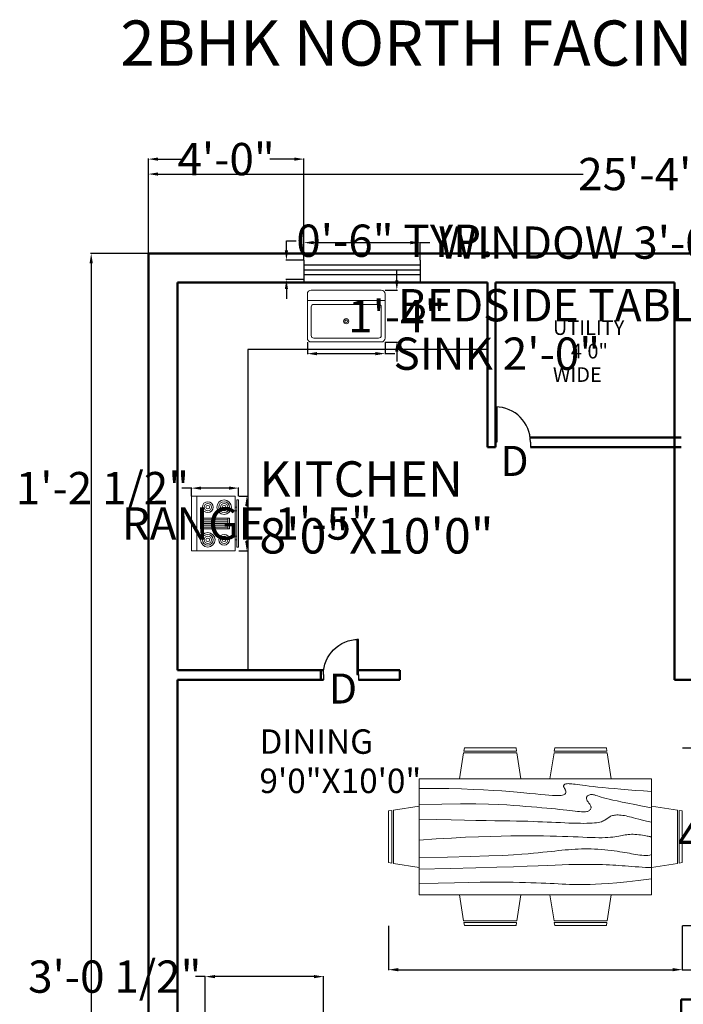
# Model space of a CAD drawing. Units: inches. Extents: x -35 to 382, y 867 to 1468.
# Tile 2 of 3: x -26 to 179, y 1163 to 1468. Entities that reach past the tile are written whole.
import ezdxf

# ---------------------------------------------------------------- set-up
doc = ezdxf.new("R2010")
doc.units = ezdxf.units.IN
doc.header["$MEASUREMENT"] = 0
for name, color, linetype, lineweight in [('A-ANNO-DIMS', 2, 'Continuous', 18), ('A-ANNO-TEXT', 7, 'Continuous', 25), ('A-AREA-IDEN', 7, 'Continuous', 25), ('A-DOOR', 3, 'Continuous', 25), ('A-EQPM', 8, 'Continuous', 18), ('A-FLOR-CASE', 32, 'Continuous', 25), ('A-FLOR-FIXT', 9, 'Continuous', 18), ('A-FURN', 9, 'Continuous', 18), ('A-GLAZ', 4, 'Continuous', 25), ('A-WALL', 7, 'Continuous', 50)]:
    doc.layers.add(name, color=color, linetype=linetype, lineweight=lineweight)
doc.styles.get("Standard").update_dxf_attribs({"font": 'arial.ttf'})
doc.dimstyles.get("Standard").update_dxf_attribs({"dimtxt": 10, "dimasz": 3, "dimexe": 0.18, "dimexo": 0.0625, "dimgap": 0.09, "dimtad": 0, "dimtih": 1, "dimtoh": 1, "dimdec": 0, "dimzin": 0, "dimdsep": 46, "dimlunit": 3, "dimtxsty": 'Standard', "dimcen": 0.09, "dimadec": 0, "dimazin": 0, "dimtfac": 1, "dimtdec": 0, "dimtofl": 0, "dimtmove": 0, "dimatfit": 3, "dimfxl": 1, "dimtolj": 1, "dimtzin": 0, "dimarcsym": 0})

# ---------------------------------------------------------------- blocks, each defined once
blk = doc.blocks.new('Sink-single - 30 in top')
blk.add_line((-15, -3.999996), (15, -3.999996))
for points in [[(-13.5, 0), (13.5, 0)], [(-15, -18.499996), (-15, -1.5)], [(15, -1.5), (15, -18.499996)], [(-13.5, -17.499996), (-13.5, -6.499996)], [(-12.5, -5.499996), (12.5, -5.499996)], [(13.5, -6.499996), (13.5, -17.499996)], [(12.5, -18.499996), (-12.5, -18.499996)], [(13.5, -19.999996), (-13.5, -19.999996)]]:
    blk.add_lwpolyline(points)
for radius in [1, 0.5]:
    blk.add_circle((0, -11.999996), radius)
for centre, radius, start, end in [((-13.5, -1.5), 1.5, 90, 180), ((13.5, -1.5), 1.5, 0, 90), ((-12.5, -6.499996), 1, 90, 180), ((12.5, -6.499996), 1, 0, 90), ((-13.5, -18.499996), 1.5, 180, 270), ((-12.5, -17.499996), 1, 180, 270), ((12.5, -17.499996), 1, 270, 0), ((13.5, -18.499996), 1.5, 270, 0)]:
    blk.add_arc(centre, radius, start, end)
blk = doc.blocks.new('Range-Oven - 30 in top')
for p, q in [((0, -3), (30, -3)), ((12, -6), (18, -6)), ((13, -20), (13, -6)), ((14, -6), (14, -20)), ((15, -20), (15, -6)), ((16, -6), (16, -20)), ((17, -20), (17, -6)), ((18, -20), (12, -20)), ((6, -24), (6, -25)), ((8, -25), (8, -24)), ((22, -25), (22, -24)), ((24, -24), (24, -25))]:
    blk.add_line(p, q)
for points in [[(0, -24), (0, 0), (30, 0), (30, -24)], [(12, -21), (12, -5), (18, -5), (18, -21)], [(2, -26), (2, -25), (28, -25), (28, -26)]]:
    blk.add_lwpolyline(points, close=True)
for centre, radius in [((6, -9), 4), ((6, -9), 3), ((6, -9), 2), ((6, -9), 1), ((24, -9), 3), ((24, -9), 2), ((24, -9), 1), ((6, -18), 3), ((6, -18), 2), ((24, -18), 4), ((24, -18), 3), ((24, -18), 2), ((6, -18), 1), ((24, -18), 1)]:
    blk.add_circle(centre, radius)
blk = doc.blocks.new('*U9')
for p, q in [((0, 0), (0, -6)), ((40, 0), (40, -6))]:
    blk.add_line(p, q)
blk.add_lwpolyline([(0, 0), (0, 40), (1.75, 40), (1.75, 0)], close=True)
blk.add_arc((0, 0), 40, 0, 90)
blk = doc.blocks.new('Dining Set - 36 x 72 in.')
for p, q in [((-22, 27.5), (-22.1562, 26.50042)), ((-22, 27.5), (-6, 27.5)), ((-5.8437, 26.49966), (-6, 27.5)), ((6, 27.5), (5.8438, 26.50042)), ((6, 27.5), (22, 27.5)), ((22.1563, 26.49966), (22, 27.5)), ((-22.2343, 26.00059), (-23.4847, 17.99762)), ((-22.2304, 26), (-5.7608, 26)), ((-5.8416, 26.5), (-22.1534, 26.5)), ((-4.5152, 17.99762), (-5.7655, 25.99926)), ((5.7657, 26.00059), (4.5153, 17.99762)), ((5.7696, 26), (22.2392, 26)), ((22.1584, 26.5), (5.8466, 26.5)), ((23.4848, 17.99762), (22.2345, 25.99926)), ((36, 18), (-36, 18)), ((-36, 18), (-36, -18)), ((36, -18), (36, 18)), ((-44.0006, 8.23428), (-35.9976, 9.48474)), ((44.0006, 8.23428), (35.9976, 9.48474)), ((-45.5, 8), (-44.5004, 8.15617)), ((-45.5, 8), (-45.5, -8)), ((-44.5, -8.15843), (-44.5, 8.15338)), ((-44, 8.23041), (-44, -8.23915)), ((44, 8.23041), (44, -8.23915)), ((44.5, -8.15843), (44.5, 8.15338)), ((45.5, 8), (44.5005, 8.15617)), ((45.5, 8), (45.5, -8)), ((-44.4997, -8.15631), (-45.5, -8)), ((-35.9976, -9.48476), (-43.9993, -8.2345)), ((35.9976, -9.48476), (43.9993, -8.2345)), ((44.4997, -8.15631), (45.5, -8)), ((-36, -18), (36, -18)), ((-22.2343, -26.0006), (-23.4847, -17.99762)), ((-4.5152, -17.99762), (-5.7655, -25.99928)), ((5.7657, -26.0006), (4.5153, -17.99762)), ((23.4848, -17.99762), (22.2345, -25.99928)), ((-22.2304, -26), (-5.7608, -26)), ((-22, -27.5), (-22.1562, -26.50044)), ((-5.8416, -26.5), (-22.1534, -26.5)), ((-5.8437, -26.49967), (-6, -27.5)), ((5.7696, -26), (22.2392, -26)), ((6, -27.5), (5.8438, -26.50044)), ((22.1584, -26.5), (5.8466, -26.5)), ((22.1563, -26.49967), (22, -27.5)), ((-22, -27.5), (-6, -27.5)), ((6, -27.5), (22, -27.5))]:
    blk.add_line(p, q)
for points in [[(-36, 15), (-31.1772, 14.97754), (-26.8079, 14.91406), (-22.8538, 14.81543), (-19.276, 14.6875), (-16.0362, 14.53613), (-13.0957, 14.36718), (-10.4159, 14.18652), (-7.9583, 14), (-5.6904, 13.81315), (-3.6035, 13.63021), (-1.6954, 13.45508), (0.0365, 13.29166), (1.5945, 13.14388), (2.9811, 13.01562), (4.1988, 12.9108), (5.25, 12.83333), (6.1393, 12.78613), (6.8802, 12.76823), (7.4883, 12.77767), (7.9792, 12.8125), (8.3685, 12.87077), (8.6719, 12.95052), (8.9049, 13.0498), (9.0833, 13.16666), (9.2205, 13.29899), (9.3216, 13.44401), (9.3895, 13.59879), (9.4271, 13.76041), (9.4373, 13.92594), (9.4232, 14.09245), (9.3875, 14.257), (9.3333, 14.41666), (9.2638, 14.56917), (9.1836, 14.71484), (9.0975, 14.85465), (9.0104, 14.98958), (8.9272, 15.1206), (8.8529, 15.2487), (8.7922, 15.37483), (8.75, 15.5), (8.7305, 15.62467), (8.7344, 15.74739), (8.7617, 15.86621), (8.8125, 15.97916), (8.8867, 16.08431), (8.9844, 16.17968), (9.1055, 16.26334), (9.25, 16.33333), (9.4189, 16.38802), (9.6172, 16.42708), (9.8506, 16.45052), (10.125, 16.45833), (10.4463, 16.45052), (10.8203, 16.42708), (11.2529, 16.38802), (11.75, 16.33333), (12.3184, 16.26318), (12.9694, 16.17838), (13.7151, 16.07991), (14.5677, 15.96875), (15.5395, 15.84586), (16.6426, 15.71224), (17.8893, 15.56884), (19.2917, 15.41666), (20.859, 15.25667), (22.5879, 15.08984), (24.4721, 14.91715), (26.5052, 14.73958), (28.6809, 14.5581), (30.9929, 14.3737), (33.4347, 14.18733), (36, 14)], [(-36, 10), (-28.9766, 10.14274), (-23.1725, 10.20442), (-18.4241, 10.19775), (-14.5677, 10.13541), (-11.4399, 10.03011), (-8.877, 9.89453), (-6.7154, 9.74137), (-4.7917, 9.58333), (-2.9698, 9.43082), (-1.2246, 9.28515), (0.4415, 9.14534), (2.026, 9.01041), (3.5266, 8.87939), (4.9408, 8.7513), (6.266, 8.62516), (7.5, 8.5), (8.6411, 8.37549), (9.6914, 8.2539), (10.6538, 8.13818), (11.5312, 8.03125), (12.3267, 7.93603), (13.043, 7.85547), (13.6831, 7.79248), (14.25, 7.75), (14.7471, 7.7303), (15.1797, 7.73307), (15.5537, 7.75732), (15.875, 7.80208), (16.1494, 7.86637), (16.3828, 7.94922), (16.5811, 8.04964), (16.75, 8.16666), (16.8944, 8.29915), (17.0143, 8.44531), (17.1089, 8.60319), (17.1771, 8.77083), (17.218, 8.94629), (17.2305, 9.1276), (17.2137, 9.31282), (17.1667, 9.5), (17.0895, 9.6875), (16.987, 9.875), (16.8649, 10.0625), (16.7292, 10.25), (16.5856, 10.4375), (16.4401, 10.625), (16.2985, 10.8125), (16.1667, 11), (16.05, 11.18733), (15.9518, 11.3737), (15.8752, 11.5581), (15.8229, 11.73958), (15.798, 11.91715), (15.8034, 12.08984), (15.842, 12.25667), (15.9167, 12.41666), (16.0295, 12.56836), (16.1784, 12.70833), (16.3605, 12.83268), (16.5729, 12.9375), (16.8127, 13.01888), (17.0768, 13.07291), (17.3625, 13.0957), (17.6667, 13.08333), (17.9894, 13.03312), (18.3418, 12.94726), (18.7382, 12.82918), (19.1927, 12.68229), (19.7195, 12.51001), (20.3327, 12.31575), (21.0465, 12.10294), (21.875, 11.875), (22.8357, 11.63354), (23.959, 11.37304), (25.2786, 11.08618), (26.8282, 10.76562), (28.6414, 10.40405), (30.752, 9.99414), (33.1936, 9.52856), (36, 9)], [(-36, 5.5), (-30.7157, 5.3348), (-26.069, 5.20963), (-21.9946, 5.11767), (-18.4271, 5.05208), (-15.3009, 5.00602), (-12.5508, 4.97265), (-10.1112, 4.94515), (-7.9167, 4.91666), (-5.909, 4.88167), (-4.0586, 4.83984), (-2.3429, 4.79215), (-0.7396, 4.73958), (0.7739, 4.6831), (2.22, 4.6237), (3.6213, 4.56233), (5, 4.5), (6.373, 4.43782), (7.7344, 4.3776), (9.0723, 4.32129), (10.375, 4.27083), (11.6309, 4.22819), (12.8281, 4.19531), (13.9551, 4.17415), (15, 4.16666), (15.954, 4.17448), (16.819, 4.19791), (17.6001, 4.23698), (18.3021, 4.29166), (18.9299, 4.36198), (19.4883, 4.44791), (19.9823, 4.54948), (20.4167, 4.66666), (20.7969, 4.79899), (21.1302, 4.94401), (21.4245, 5.09879), (21.6875, 5.26041), (21.9271, 5.42594), (22.1511, 5.59245), (22.3672, 5.757), (22.5834, 5.91666), (22.8065, 6.06868), (23.0404, 6.21093), (23.2879, 6.34147), (23.5521, 6.45833), (23.8358, 6.55957), (24.142, 6.64323), (24.4735, 6.70735), (24.8334, 6.75), (25.2235, 6.76969), (25.642, 6.76692), (26.0858, 6.74267), (26.5521, 6.69791), (27.0379, 6.63362), (27.5404, 6.55078), (28.0565, 6.45036), (28.5834, 6.33333), (29.1242, 6.19987), (29.7071, 6.04687), (30.3661, 5.87044), (31.1354, 5.66666), (32.0493, 5.43164), (33.142, 5.16146), (34.4475, 4.85221), (36, 4.5)], [(-36, -1), (-30.7915, -0.6591), (-26.0195, -0.38216), (-21.6519, -0.16284), (-17.6563, 0.00521), (-14.0005, 0.12833), (-10.6523, 0.21289), (-7.5796, 0.26522), (-4.75, 0.29166), (-2.134, 0.29793), (0.2878, 0.28711), (2.5317, 0.26163), (4.6146, 0.22396), (6.5529, 0.17651), (8.3633, 0.12174), (10.0623, 0.06209), (11.6667, 0), (13.1899, -0.06201), (14.6341, -0.1211), (15.9982, -0.17432), (17.2813, -0.21875), (18.4823, -0.25147), (19.6003, -0.26953), (20.6343, -0.27002), (21.5834, -0.25), (22.4481, -0.20768), (23.2357, -0.14584), (23.9549, -0.06836), (24.6146, 0.02083), (25.2235, 0.11784), (25.7904, 0.21875), (26.3241, 0.31966), (26.8334, 0.41666), (27.3265, 0.50618), (27.8099, 0.58593), (28.2894, 0.65397), (28.7709, 0.70833), (29.2601, 0.74707), (29.763, 0.76823), (30.2855, 0.76985), (30.8334, 0.75), (31.4088, 0.70784), (31.9994, 0.64713), (32.589, 0.57275), (33.1615, 0.48958), (33.7008, 0.4025), (34.1908, 0.3164), (34.6153, 0.23616), (34.9584, 0.16666), (35.2099, 0.11165), (35.3848, 0.07031), (35.504, 0.04069), (35.5886, 0.02083), (35.6594, 0.00879), (35.7377, 0.0026), (35.8442, 0.00032), (36, 0)], [(-36, -6.5), (-27.1843, -6.31267), (-20.084, -6.1263), (-14.469, -5.9419), (-10.1094, -5.76042), (-6.7752, -5.58285), (-4.2363, -5.41016), (-2.2629, -5.24333), (-0.625, -5.08334), (0.8708, -4.93099), (2.2715, -4.78646), (3.5872, -4.64974), (4.8281, -4.52084), (6.0046, -4.39974), (7.127, -4.28646), (8.2053, -4.18099), (9.25, -4.08334), (10.2705, -3.99382), (11.2734, -3.91407), (12.2647, -3.84603), (13.25, -3.79167), (14.2354, -3.75293), (15.2266, -3.73177), (16.2295, -3.73015), (17.25, -3.75), (18.2912, -3.79248), (19.3451, -3.85547), (20.4009, -3.93604), (21.4479, -4.03125), (22.4754, -4.13819), (23.4727, -4.25391), (24.4289, -4.37549), (25.3334, -4.5), (26.1785, -4.62492), (26.9694, -4.74935), (27.7145, -4.87281), (28.4219, -4.99479), (29.1, -5.11483), (29.7572, -5.23242), (30.4016, -5.34709), (31.0417, -5.45834), (31.6837, -5.56437), (32.3262, -5.65821), (32.9658, -5.73153), (33.599, -5.77604), (34.2224, -5.78345), (34.8327, -5.74545), (35.4264, -5.65373), (36, -5.5)], [(-36, -10), (-26.4022, -9.81299), (-18.4675, -9.62891), (-11.9839, -9.45069), (-6.7396, -9.28125), (-2.5226, -9.12354), (0.8789, -8.98047), (3.6769, -8.85498), (6.0833, -8.75), (8.2767, -8.66765), (10.3021, -8.60677), (12.1712, -8.56543), (13.8958, -8.54167), (15.4876, -8.53353), (16.9583, -8.53907), (18.3197, -8.55632), (19.5834, -8.58334), (20.7616, -8.61841), (21.8685, -8.66081), (22.9188, -8.71004), (23.9271, -8.76563), (24.9081, -8.82707), (25.8763, -8.89388), (26.8465, -8.96558), (27.8334, -9.04167), (28.8474, -9.12118), (29.8828, -9.20117), (30.93, -9.27824), (31.9792, -9.34896), (33.0205, -9.40991), (34.0443, -9.45768), (35.0407, -9.48885), (36, -9.5)], [(-36, -14.5), (-30.0881, -14.33513), (-25.0332, -14.21224), (-20.7312, -14.12647), (-17.0781, -14.07292), (-13.97, -14.04671), (-11.3027, -14.04297), (-8.9724, -14.05681), (-6.875, -14.08334), (-4.9224, -14.11833), (-3.0905, -14.16016), (-1.3709, -14.20785), (0.2448, -14.26042), (1.7647, -14.3169), (3.1973, -14.3763), (4.5507, -14.43767), (5.8333, -14.5), (7.0554, -14.5621), (8.235, -14.62175), (9.3922, -14.67652), (10.5469, -14.72396), (11.7192, -14.76164), (12.929, -14.78711), (14.1965, -14.79794), (15.5417, -14.79167), (16.9933, -14.76424), (18.6152, -14.70508), (20.4804, -14.60197), (22.6615, -14.44271), (25.2312, -14.21509), (28.2624, -13.9069), (31.8277, -13.50594), (36, -13)]]:
    blk.add_lwpolyline(points)
blk = doc.blocks.new('Window - Wood Frame 36 in. Wide plan')
for p, q in [((0, 6), (0, 0)), ((0, 4.5), (36, 4.5)), ((36, 6), (36, 0)), ((0, 3), (36, 3)), ((0, 1.5), (36, 1.5))]:
    blk.add_line(p, q)
blk = doc.blocks.new('*D15')
at = {"layer": 'A-ANNO-DIMS', "color": 0, "lineweight": -2, "transparency": 16777216}
for p, q in [((13.52, 1395.38), (13.52, 1420.11)), ((16.52, 1419.93), (148.17, 1419.93)), ((314.52, 1419.93), (182.87, 1419.93)), ((317.52, 1395.38), (317.52, 1420.11))]:
    blk.add_line(p, q, dxfattribs=at)
at = {"layer": 'A-ANNO-DIMS', "color": 0, "transparency": 16777216}
for points in [[(16.52, 1420.43), (16.52, 1419.43), (13.52, 1419.93)], [(314.52, 1420.43), (314.52, 1419.43), (317.52, 1419.93)]]:
    blk.add_solid(points, dxfattribs=at)
at = {"layer": 'Defpoints', "color": 0, "transparency": 16777216}
for p in [(317.52, 1419.93), (13.52, 1395.31), (317.52, 1395.31)]:
    blk.add_point(p, dxfattribs=at)
at = {"layer": 'A-ANNO-DIMS', "color": 0, "transparency": 16777216, "insert": (165.52, 1419.93), "char_height": 10, "attachment_point": 5}
blk.add_mtext('\\A1;25\'-4"', dxfattribs=at)
blk = doc.blocks.new('*D16')
at = {"layer": 'A-ANNO-DIMS', "color": 0, "lineweight": -2, "transparency": 16777216}
for p, q in [((13.46, 1395.31), (-4.36, 1395.31)), ((-4.18, 1392.31), (-4.18, 1158.51)), ((-4.18, 914.31), (-4.18, 1148.12)), ((13.46, 911.31), (-4.36, 911.31))]:
    blk.add_line(p, q, dxfattribs=at)
at = {"layer": 'A-ANNO-DIMS', "color": 0, "transparency": 16777216}
for points in [[(-4.68, 1392.31), (-3.68, 1392.31), (-4.18, 1395.31)], [(-4.68, 914.31), (-3.68, 914.31), (-4.18, 911.31)]]:
    blk.add_solid(points, dxfattribs=at)
at = {"layer": 'Defpoints', "color": 0, "transparency": 16777216}
for p in [(13.52, 1395.31), (-4.18, 911.31), (13.52, 911.31)]:
    blk.add_point(p, dxfattribs=at)
at = {"layer": 'A-ANNO-DIMS', "color": 0, "transparency": 16777216, "insert": (-4.18, 1153.31), "char_height": 10, "attachment_point": 5}
blk.add_mtext('\\A1;40\'-4"', dxfattribs=at)
blk = doc.blocks.new('*D18')
at = {"layer": 'A-ANNO-DIMS', "color": 0, "lineweight": -2, "transparency": 16777216}
for p, q in [((61.69, 1393.35), (61.69, 1398.87)), ((64.69, 1398.69), (94.69, 1398.69)), ((97.69, 1393.35), (97.69, 1398.87)), ((97.69, 1398.69), (100.69, 1398.69))]:
    blk.add_line(p, q, dxfattribs=at)
at = {"layer": 'A-ANNO-DIMS', "color": 0, "transparency": 16777216}
for points in [[(64.69, 1399.19), (64.69, 1398.19), (61.69, 1398.69)], [(94.69, 1399.19), (94.69, 1398.19), (97.69, 1398.69)]]:
    blk.add_solid(points, dxfattribs=at)
at = {"layer": 'Defpoints', "color": 0, "transparency": 16777216}
for p in [(97.69, 1398.69), (61.69, 1393.29), (97.69, 1393.29)]:
    blk.add_point(p, dxfattribs=at)
at = {"layer": 'A-ANNO-DIMS', "color": 0, "transparency": 16777216, "insert": (164.05, 1398.69), "char_height": 10, "attachment_point": 5}
blk.add_mtext('\\A1;WINDOW 3\'-0" TYP.', dxfattribs=at)
blk = doc.blocks.new('*D19')
at = {"layer": 'A-ANNO-DIMS', "color": 0, "lineweight": -2, "transparency": 16777216}
for p, q in [((56.29, 1396.29), (56.29, 1399.29)), ((56.29, 1399.29), (59.29, 1399.29)), ((61.63, 1393.29), (56.11, 1393.29)), ((61.63, 1387.29), (56.11, 1387.29)), ((56.29, 1384.29), (56.29, 1381.29))]:
    blk.add_line(p, q, dxfattribs=at)
at = {"layer": 'A-ANNO-DIMS', "color": 0, "transparency": 16777216}
for points in [[(55.79, 1396.29), (56.79, 1396.29), (56.29, 1393.29)], [(55.79, 1384.29), (56.79, 1384.29), (56.29, 1387.29)]]:
    blk.add_solid(points, dxfattribs=at)
at = {"layer": 'Defpoints', "color": 0, "transparency": 16777216}
for p in [(56.29, 1393.29), (61.69, 1393.29), (61.69, 1387.29)]:
    blk.add_point(p, dxfattribs=at)
at = {"layer": 'A-ANNO-DIMS', "color": 0, "transparency": 16777216, "insert": (89.86, 1399.29), "char_height": 10, "attachment_point": 5}
blk.add_mtext('\\A1;0\'-6" TYP.', dxfattribs=at)
blk = doc.blocks.new('*D22')
at = {"layer": 'A-ANNO-DIMS', "color": 0, "lineweight": -2, "transparency": 16777216}
for p, q in [((286.27, 1379.31), (283.27, 1379.31)), ((286.27, 1377.52), (286.27, 1379.49)), ((295.61, 1379.31), (289.27, 1379.31)), ((298.61, 1377.52), (298.61, 1379.49))]:
    blk.add_line(p, q, dxfattribs=at)
at = {"layer": 'A-ANNO-DIMS', "color": 0, "transparency": 16777216}
for points in [[(289.27, 1379.81), (289.27, 1378.81), (286.27, 1379.31)], [(295.61, 1379.81), (295.61, 1378.81), (298.61, 1379.31)]]:
    blk.add_solid(points, dxfattribs=at)
at = {"layer": 'Defpoints', "color": 0, "transparency": 16777216}
for p in [(286.27, 1379.31), (286.27, 1377.46), (298.61, 1377.46)]:
    blk.add_point(p, dxfattribs=at)
at = {"layer": 'A-ANNO-DIMS', "color": 0, "transparency": 16777216, "insert": (184.6, 1379.31), "char_height": 10, "attachment_point": 5}
blk.add_mtext('\\A1;BEDSIDE TABLE 1\'-0 1/2" TYP.', dxfattribs=at)
blk = doc.blocks.new('*D31')
at = {"layer": 'A-ANNO-DIMS', "color": 0, "lineweight": -2, "transparency": 16777216}
for p, q in [((31.15, 1171.39), (28.15, 1171.39)), ((31.15, 1158.85), (31.15, 1171.57)), ((64.82, 1171.39), (34.15, 1171.39)), ((67.82, 1158.85), (67.82, 1171.57))]:
    blk.add_line(p, q, dxfattribs=at)
at = {"layer": 'A-ANNO-DIMS', "color": 0, "transparency": 16777216}
for points in [[(34.15, 1171.89), (34.15, 1170.89), (31.15, 1171.39)], [(64.82, 1171.89), (64.82, 1170.89), (67.82, 1171.39)]]:
    blk.add_solid(points, dxfattribs=at)
at = {"layer": 'Defpoints', "color": 0, "transparency": 16777216}
for p in [(31.15, 1171.39), (31.15, 1158.79), (67.82, 1158.79)]:
    blk.add_point(p, dxfattribs=at)
at = {"layer": 'A-ANNO-DIMS', "color": 0, "transparency": 16777216, "insert": (3.12, 1171.39), "char_height": 10, "attachment_point": 5}
blk.add_mtext('\\A1;3\'-0 1/2"', dxfattribs=at)
blk = doc.blocks.new('*D32')
at = {"layer": 'A-ANNO-DIMS', "color": 0, "lineweight": -2, "transparency": 16777216}
for p, q in [((62.77, 1367.86), (62.77, 1364.13)), ((86.86, 1367.86), (86.86, 1364.13)), ((65.77, 1364.31), (83.86, 1364.31)), ((86.86, 1364.31), (89.86, 1364.31))]:
    blk.add_line(p, q, dxfattribs=at)
at = {"layer": 'A-ANNO-DIMS', "color": 0, "transparency": 16777216}
for points in [[(65.77, 1364.81), (65.77, 1363.81), (62.77, 1364.31)], [(83.86, 1364.81), (83.86, 1363.81), (86.86, 1364.31)]]:
    blk.add_solid(points, dxfattribs=at)
at = {"layer": 'Defpoints', "color": 0, "transparency": 16777216}
for p in [(62.77, 1367.92), (86.86, 1367.92), (86.86, 1364.31)]:
    blk.add_point(p, dxfattribs=at)
at = {"layer": 'A-ANNO-DIMS', "color": 0, "transparency": 16777216, "insert": (121.46, 1364.31), "char_height": 10, "attachment_point": 5}
blk.add_mtext('\\A1;SINK 2\'-0"', dxfattribs=at)
blk = doc.blocks.new('*D33')
at = {"layer": 'A-ANNO-DIMS', "color": 0, "lineweight": -2, "transparency": 16777216}
for p, q in [((90.47, 1386.98), (90.47, 1389.98)), ((86.92, 1383.98), (90.65, 1383.98)), ((86.92, 1367.92), (90.65, 1367.92)), ((90.47, 1364.92), (90.47, 1361.92))]:
    blk.add_line(p, q, dxfattribs=at)
at = {"layer": 'A-ANNO-DIMS', "color": 0, "transparency": 16777216}
for points in [[(89.97, 1386.98), (90.97, 1386.98), (90.47, 1383.98)], [(89.97, 1364.92), (90.97, 1364.92), (90.47, 1367.92)]]:
    blk.add_solid(points, dxfattribs=at)
at = {"layer": 'Defpoints', "color": 0, "transparency": 16777216}
for p in [(86.86, 1383.98), (90.47, 1383.98), (86.86, 1367.92)]:
    blk.add_point(p, dxfattribs=at)
at = {"layer": 'A-ANNO-DIMS', "color": 0, "transparency": 16777216, "insert": (90.47, 1375.95), "char_height": 10, "attachment_point": 5}
blk.add_mtext('\\A1;1\'-4"', dxfattribs=at)
blk = doc.blocks.new('*D34')
at = {"layer": 'A-ANNO-DIMS', "color": 0, "lineweight": -2, "transparency": 16777216}
for p, q in [((41.54, 1320.14), (44.19, 1320.14)), ((44.01, 1317.14), (44.01, 1316.98)), ((44.01, 1306.29), (44.01, 1306.45)), ((41.54, 1303.29), (44.19, 1303.29))]:
    blk.add_line(p, q, dxfattribs=at)
at = {"layer": 'A-ANNO-DIMS', "color": 0, "transparency": 16777216}
for points in [[(43.51, 1317.14), (44.51, 1317.14), (44.01, 1320.14)], [(43.51, 1306.29), (44.51, 1306.29), (44.01, 1303.29)]]:
    blk.add_solid(points, dxfattribs=at)
at = {"layer": 'Defpoints', "color": 0, "transparency": 16777216}
for p in [(41.48, 1320.14), (44.01, 1320.14), (41.48, 1303.29)]:
    blk.add_point(p, dxfattribs=at)
at = {"layer": 'A-ANNO-DIMS', "color": 0, "transparency": 16777216, "insert": (44.01, 1311.71), "char_height": 10, "attachment_point": 5}
blk.add_mtext('\\A1;RANGE 1\'-5"', dxfattribs=at)
blk = doc.blocks.new('*D35')
at = {"layer": 'A-ANNO-DIMS', "color": 0, "lineweight": -2, "transparency": 16777216}
for p, q in [((26.88, 1322.67), (23.88, 1322.67)), ((26.88, 1320.2), (26.88, 1322.85)), ((38.48, 1322.67), (29.88, 1322.67)), ((41.48, 1320.2), (41.48, 1322.85))]:
    blk.add_line(p, q, dxfattribs=at)
at = {"layer": 'A-ANNO-DIMS', "color": 0, "transparency": 16777216}
for points in [[(29.88, 1323.17), (29.88, 1322.17), (26.88, 1322.67)], [(38.48, 1323.17), (38.48, 1322.17), (41.48, 1322.67)]]:
    blk.add_solid(points, dxfattribs=at)
at = {"layer": 'Defpoints', "color": 0, "transparency": 16777216}
for p in [(26.88, 1322.67), (26.88, 1320.14), (41.48, 1320.14)]:
    blk.add_point(p, dxfattribs=at)
at = {"layer": 'A-ANNO-DIMS', "color": 0, "transparency": 16777216, "insert": (-0.69, 1322.67), "char_height": 10, "attachment_point": 5}
blk.add_mtext('\\A1;1\'-2 1/2"', dxfattribs=at)
blk = doc.blocks.new('*D36')
at = {"layer": 'A-ANNO-DIMS', "color": 0, "lineweight": -2, "transparency": 16777216}
for p, q in [((87.91, 1187.13), (87.91, 1173.36)), ((178.91, 1187.13), (178.91, 1173.36)), ((90.91, 1173.54), (175.91, 1173.54)), ((178.91, 1173.54), (181.91, 1173.54))]:
    blk.add_line(p, q, dxfattribs=at)
at = {"layer": 'A-ANNO-DIMS', "color": 0, "transparency": 16777216}
for points in [[(90.91, 1174.04), (90.91, 1173.04), (87.91, 1173.54)], [(175.91, 1174.04), (175.91, 1173.04), (178.91, 1173.54)]]:
    blk.add_solid(points, dxfattribs=at)
at = {"layer": 'Defpoints', "color": 0, "transparency": 16777216}
for p in [(87.91, 1187.19), (178.91, 1187.19), (178.91, 1173.54)]:
    blk.add_point(p, dxfattribs=at)
at = {"layer": 'A-ANNO-DIMS', "color": 0, "transparency": 16777216, "insert": (236.96, 1173.54), "char_height": 10, "attachment_point": 5}
blk.add_mtext('\\A1;DINING SET 7\'-7"', dxfattribs=at)
blk = doc.blocks.new('*D37')
at = {"layer": 'A-ANNO-DIMS', "color": 0, "lineweight": -2, "transparency": 16777216}
for p, q in [((178.97, 1242.19), (192.74, 1242.19)), ((192.56, 1239.19), (192.56, 1219.78)), ((192.56, 1190.19), (192.56, 1209.6)), ((178.97, 1187.19), (192.74, 1187.19))]:
    blk.add_line(p, q, dxfattribs=at)
at = {"layer": 'A-ANNO-DIMS', "color": 0, "transparency": 16777216}
for points in [[(192.06, 1239.19), (193.06, 1239.19), (192.56, 1242.19)], [(192.06, 1190.19), (193.06, 1190.19), (192.56, 1187.19)]]:
    blk.add_solid(points, dxfattribs=at)
at = {"layer": 'Defpoints', "color": 0, "transparency": 16777216}
for p in [(178.91, 1242.19), (192.56, 1242.19), (178.91, 1187.19)]:
    blk.add_point(p, dxfattribs=at)
at = {"layer": 'A-ANNO-DIMS', "color": 0, "transparency": 16777216, "insert": (192.56, 1214.69), "char_height": 10, "attachment_point": 5}
blk.add_mtext('\\A1;4\'-7"', dxfattribs=at)
blk = doc.blocks.new('*D47')
at = {"layer": 'A-ANNO-DIMS', "color": 0, "lineweight": -2, "transparency": 16777216}
for p, q in [((13.52, 1395.38), (13.52, 1424.74)), ((16.52, 1424.56), (24.02, 1424.56)), ((58.69, 1424.56), (51.19, 1424.56)), ((61.69, 1395.38), (61.69, 1424.74))]:
    blk.add_line(p, q, dxfattribs=at)
at = {"layer": 'A-ANNO-DIMS', "color": 0, "transparency": 16777216}
for points in [[(16.52, 1425.06), (16.52, 1424.06), (13.52, 1424.56)], [(58.69, 1425.06), (58.69, 1424.06), (61.69, 1424.56)]]:
    blk.add_solid(points, dxfattribs=at)
at = {"layer": 'Defpoints', "color": 0, "transparency": 16777216}
for p in [(61.69, 1424.56), (13.52, 1395.31), (61.69, 1395.31)]:
    blk.add_point(p, dxfattribs=at)
at = {"layer": 'A-ANNO-DIMS', "color": 0, "transparency": 16777216, "insert": (37.61, 1424.56), "char_height": 10, "attachment_point": 5}
blk.add_mtext('\\A1;4\'-0"', dxfattribs=at)

msp = doc.modelspace()

# ---------------------------------------------------------------- linework, layer by layer
at = {"layer": 'A-FLOR-CASE'}
for p, q in [((118.52, 1365.57), (44.34, 1365.57)), ((44.34, 1365.57), (44.34, 1266.31))]:
    msp.add_line(p, q, dxfattribs=at)
at = {"layer": 'A-GLAZ'}
for p, q in [((61.69, 1393.29), (61.69, 1395.31)), ((97.69, 1393.29), (97.69, 1395.31)), ((61.69, 1387.29), (61.69, 1386.31)), ((97.69, 1387.29), (97.69, 1386.31))]:
    msp.add_line(p, q, dxfattribs=at)
at = {"layer": 'A-WALL'}
for p, q in [((13.52, 911.31), (13.52, 1395.31)), ((13.52, 1395.31), (317.52, 1395.31)), ((22.52, 1386.31), (118.52, 1386.31)), ((22.52, 1266.31), (22.52, 1386.31)), ((118.52, 1335.31), (118.52, 1386.31)), ((121.02, 1335.31), (121.02, 1386.31)), ((121.02, 1386.31), (176.52, 1386.31)), ((176.52, 1263.31), (176.52, 1386.31)), ((121.02, 1338.31), (121.5, 1338.31)), ((131.8, 1338.31), (178.52, 1338.31)), ((118.52, 1335.31), (121.02, 1335.31)), ((131.89, 1335.31), (178.52, 1335.31)), ((22.52, 1266.31), (67.81, 1266.31)), ((66.9, 1266.31), (66.9, 1263.31)), ((78.12, 1266.31), (91.43, 1266.31)), ((91.43, 1266.31), (91.43, 1263.31)), ((22.52, 1263.31), (67.73, 1263.31)), ((22.52, 1053.31), (22.52, 1263.31)), ((78.6, 1263.31), (91.43, 1263.31)), ((176.52, 1263.31), (186.49, 1263.31)), ((178.52, 1098.31), (178.52, 1164.31)), ((178.52, 1164.31), (257.52, 1164.31))]:
    msp.add_line(p, q, dxfattribs=at)

# ---------------------------------------------------------------- block references
at = {"layer": 'A-DOOR', "yscale": 0.2717391304347826, "zscale": 0.2717391304347826}
for p, xscale in [((121.02, 1336.95), 0.2717391304347826), ((78.6, 1264.95), -0.2717391304347826)]:
    msp.add_blockref('*U9', p, dxfattribs=dict(at, xscale=xscale))
at = {"layer": 'A-EQPM', "xscale": 0.5617430650316791, "yscale": 0.5617430650316791, "zscale": 0.5617430650316791, "rotation": 90}
msp.add_blockref('Range-Oven - 30 in top', (26.88, 1303.29), dxfattribs=at)
at = {"layer": 'A-FLOR-FIXT', "xscale": 0.8027729719194864, "yscale": 0.8027729719194864, "zscale": 0.8027729719194864}
msp.add_blockref('Sink-single - 30 in top', (74.81, 1383.98), dxfattribs=at)
at = {"layer": 'A-FURN'}
msp.add_blockref('Dining Set - 36 x 72 in.', (133.41, 1214.69), dxfattribs=at)
at = {"layer": 'A-GLAZ'}
msp.add_blockref('Window - Wood Frame 36 in. Wide plan', (61.69, 1387.29), dxfattribs=at)

# ---------------------------------------------------------------- texts
at = {"layer": 'A-ANNO-TEXT'}
for s, height, p in [('2BHK NORTH FACING HOUSE PLAN', 14.0085, (4.86, 1453.48)), ('D', 9.31, (122.56, 1326.43)), ('D', 9.31, (69.44, 1255.95))]:
    msp.add_text(s, height=height, dxfattribs=at).set_placement(p)
at = {"layer": 'A-AREA-IDEN'}
for s, height, p in [('UTILITY', 4.529, (138.83, 1370.11)), ('    4\'0"', 4.529, (138.83, 1362.83)), ('WIDE', 4.529, (138.83, 1355.56)), ('KITCHEN', 10.958, (47.92, 1320.02)), ('8\'0"X10\'0"', 10.958, (47.92, 1302.42)), ('DINING ', 7.57, (47.94, 1240.39)), ('9\'0"X10\'0"', 7.57, (47.94, 1228.23))]:
    msp.add_text(s, height=height, dxfattribs=at).set_placement(p)

# ---------------------------------------------------------------- dimensions: what is measured, and where the dimension line sits
at = {"layer": 'A-ANNO-DIMS'}
for base, p2, override, picture, middle in [((61.69, 1424.56), (61.69, 1395.31), {"dimdec": 1, "dimlfac": 1, "dimrnd": 0, "dimzin": 1, "dimdsep": 46, "dimlunit": 4, "dimfrac": 2}, '*D47', (37.61, 1424.56)), ((317.52, 1419.93), (317.52, 1395.31), {"dimclrd": 0, "dimclre": 0, "dimclrt": 0}, '*D15', (165.52, 1419.93))]:
    dim = msp.add_linear_dim(base=base, p1=(13.52, 1395.31), p2=p2, dimstyle='Standard', override=override, dxfattribs=at)
    dim.commit()
    dim.dimension.update_dxf_attribs({"geometry": picture, "text_midpoint": middle})
for base, p1, p2, text, picture, middle in [((97.69, 1398.69), (61.69, 1393.29), (97.69, 1393.29), 'WINDOW <> TYP.', '*D18', (164.05, 1398.69)), ((86.86, 1364.31), (62.77, 1367.92), (86.86, 1367.92), 'SINK <>', '*D32', (121.46, 1364.31)), ((178.91, 1173.54), (87.91, 1187.19), (178.91, 1187.19), 'DINING SET <>', '*D36', (236.96, 1173.54))]:
    dim = msp.add_linear_dim(base=base, p1=p1, p2=p2, text=text, dimstyle='Standard', override={"dimdec": 1, "dimlfac": 1, "dimrnd": 0, "dimzin": 1, "dimdsep": 46, "dimlunit": 4, "dimfrac": 2}, dxfattribs=at)
    dim.commit()
    dim.dimension.update_dxf_attribs({"geometry": picture, "text_midpoint": middle})
for base, p1, p2, angle, text, picture, middle in [((286.27, 1379.31), (298.61, 1377.46), (286.27, 1377.46), 180, 'BEDSIDE TABLE <> TYP.', '*D22', (184.6, 1379.31)), ((56.29, 1393.29), (61.69, 1387.29), (61.69, 1393.29), 90, '<> TYP.', '*D19', (89.86, 1399.29)), ((44.009, 1320.1406), (41.4812, 1303.2884), (41.4812, 1320.1406), 90, 'RANGE <>', '*D34', (44.009, 1311.7145))]:
    dim = msp.add_linear_dim(base=base, p1=p1, p2=p2, angle=angle, text=text, dimstyle='Standard', override={"dimdec": 1, "dimlfac": 1, "dimrnd": 0, "dimzin": 1, "dimdsep": 46, "dimlunit": 4, "dimfrac": 2}, dxfattribs=at)
    dim.commit()
    dim.dimension.update_dxf_attribs({"geometry": picture, "text_midpoint": middle})
for base, p1, p2, angle, override, picture, middle in [((-4.18, 911.31), (13.52, 1395.31), (13.52, 911.31), 90, {"dimclrd": 0, "dimclre": 0, "dimclrt": 0}, '*D16', (-4.18, 1153.31)), ((90.47, 1383.98), (86.86, 1367.92), (86.86, 1383.98), 90, {"dimdec": 1, "dimlfac": 1, "dimrnd": 0, "dimzin": 1, "dimdsep": 46, "dimlunit": 4, "dimfrac": 2}, '*D33', (90.47, 1375.95)), ((26.88, 1322.67), (41.48, 1320.14), (26.88, 1320.14), 180, {"dimdec": 1, "dimlfac": 1, "dimrnd": 0, "dimzin": 1, "dimdsep": 46, "dimlunit": 4, "dimfrac": 2}, '*D35', (-0.69, 1322.67)), ((192.56, 1242.19), (178.91, 1187.19), (178.91, 1242.19), 90, {"dimdec": 1, "dimlfac": 1, "dimrnd": 0, "dimzin": 1, "dimdsep": 46, "dimlunit": 4, "dimfrac": 2}, '*D37', (192.56, 1214.69)), ((31.15, 1171.39), (67.82, 1158.79), (31.15, 1158.79), 180, {"dimdec": 1, "dimlfac": 1, "dimrnd": 0, "dimzin": 1, "dimdsep": 46, "dimlunit": 4, "dimfrac": 2}, '*D31', (3.12, 1171.39))]:
    dim = msp.add_linear_dim(base=base, p1=p1, p2=p2, angle=angle, dimstyle='Standard', override=override, dxfattribs=at)
    dim.commit()
    dim.dimension.update_dxf_attribs({"geometry": picture, "text_midpoint": middle})

doc.saveas('drawing.dxf')
